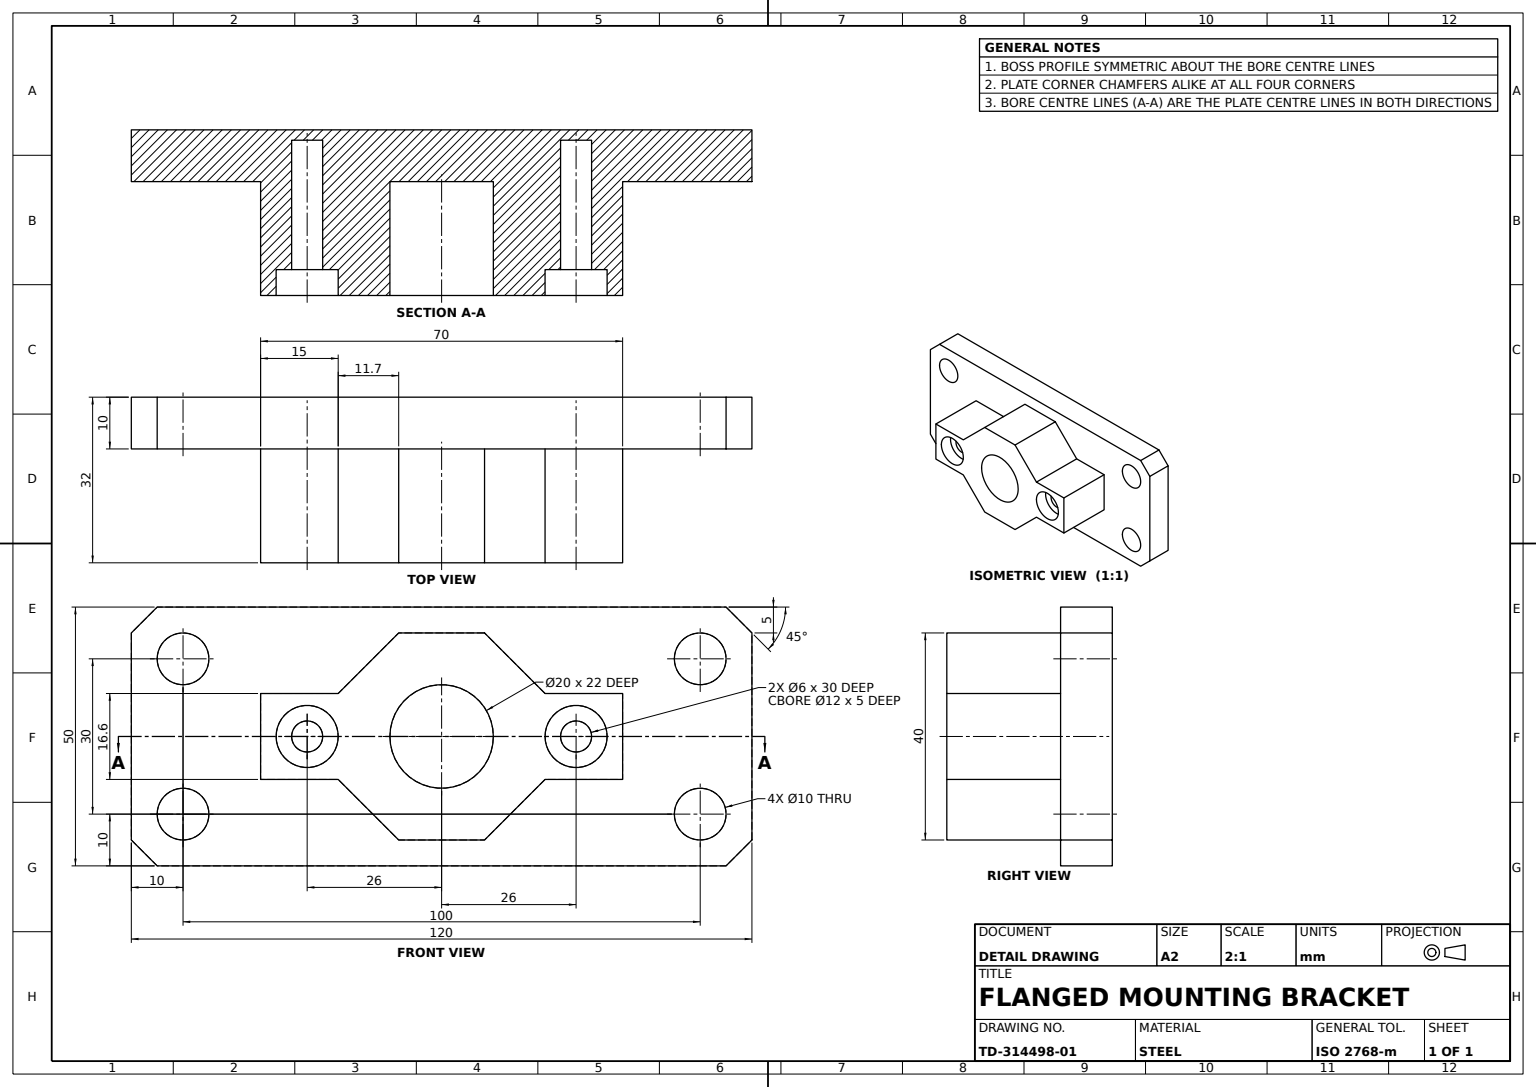
SolidWorks part; units mm, degrees
material "Plain Carbon Steel"
ref_plane "Front Plane" through (0, 0, 0) normal (0, 0, 1) x (1, 0, 0)
ref_plane "Top Plane" through (0, 0, 0) normal (0, 1, 0) x (1, 0, 0)
ref_plane "Right Plane" through (0, 0, 0) normal (1, 0, 0) x (0, 0, -1)
sketch "Base Plate Sketch" plane through (0, 0, 0) normal (0, 0, 1) x (1, 0, 0)
  line L1 (-60, 25) -> (60, 25)
  line L2 (-60, 25) -> (-60, -25)
  line L3 (-60, -25) -> (60, -25)
  line L4 (60, 25) -> (60, -25)
  line L5 (-60, 25) -> (60, -25) construction
  line L6 (-60, -25) -> (60, 25) construction
  point P0 (0, 0)
  dimension "D1" = 120
  dimension "D2" = 50
extrude "Base Plate 120x50x10" add sketch "Base Plate Sketch" along normal blind 10
sketch "Clamp Boss Sketch" plane through (0, 0, 10) normal (0, 0, 1) x (1, 0, 0)
  line L0 (20, 8.3) -> (35, 8.3)
  line L2 (20, 8.3) -> (8.3, 20)
  line L3 (8.3, 20) -> (-8.3, 20)
  line L4 (-8.3, 20) -> (-20, 8.3)
  line L6 (-20, -8.3) -> (-8.3, -20)
  line L7 (-8.3, -20) -> (8.3, -20)
  line L8 (8.3, -20) -> (20, -8.3)
  line L9 (-35, 8.3) -> (-20, 8.3)
  line L10 (-35, 8.3) -> (-35, -8.3)
  line L11 (-35, -8.3) -> (-20, -8.3)
  line L12 (35, 8.3) -> (35, -8.3)
  line L13 (-35, 8.3) -> (35, -8.3) construction
  line L14 (-35, -8.3) -> (35, 8.3) construction
  line L15 (20, -8.3) -> (35, -8.3)
  line L16 (-88.7143, 0) -> (80.2025, 0) construction
  line L17 (0, 43.4762) -> (0, -48.9359) construction
  point P0 (0, 20)
  point P16 (-35, 0)
  dimension "D1" = 16.6
  dimension "D2" = 16.6
  dimension "D3" = 70
  dimension "D4" = 15
  dimension "D5" = 15
  dimension "D6" = 15
  dimension "D7" = 15
  dimension "D8" = 11.7
  dimension "D9" = 16.6
  dimension "D10" = 11.7
  dimension "D11" = 20
  dimension "D12" = 20
  dimension "D13" = 11.7
extrude "Clamp Boss" add sketch "Clamp Boss Sketch" along normal blind 22 contours L4 L9 L10 L11 L6 L7 L8 L15 L12 L0 L2 L3
sketch "Bore Sketch" plane through (0, 0, 32) normal (0, 0, 1) x (1, 0, 0)
  circle A0 centre (0, 0) radius 10
  dimension "D1" = 20
extrude "Bore Ø20" cut sketch "Bore Sketch" against normal blind 22
sketch "Counterbore Sketch" plane through (0, 0, 32) normal (0, 0, 1) x (1, 0, 0)
  circle A0 centre (-26, 0) radius 6
  circle A1 centre (26, 0) radius 6
  dimension "D1" = 12
  dimension "D2" = 26
  dimension "D3" = 26
extrude "Counterbores 2xØ12" cut sketch "Counterbore Sketch" against normal blind 5
sketch "Bolt Hole Sketch" plane through (0, 0, 27) normal (0, 0, 1) x (1, 0, 0)
  circle A0 centre (-26, 0) radius 3
  circle A1 centre (26, 0) radius 3
  dimension "D1" = 6
  dimension "D2" = 6
  dimension "D3" = 26
  dimension "D4" = 26
extrude "Bolt Holes 2xØ6" cut sketch "Bolt Hole Sketch" against normal blind 25
sketch "Mounting Hole Sketch" plane through (0, 0, 10) normal (0, 0, 1) x (1, 0, 0)
  circle A0 centre (50, 15) radius 5
  circle A1 centre (50, -15) radius 5
  circle A2 centre (-50, 15) radius 5
  circle A3 centre (-50, -15) radius 5
  dimension "D1" = 10
  dimension "D2" = 10
  dimension "D3" = 15
  dimension "D4" = 50
  dimension "D5" = 50
extrude "Mounting Holes 4xØ10" cut sketch "Mounting Hole Sketch" against normal blind 25
chamfer "Corner Chamfers 5mm" distance 5 angle 45 4 edges at (60, -25, 5) (-60, -25, 5) (-60, 25, 5) (60, 25, 5)
